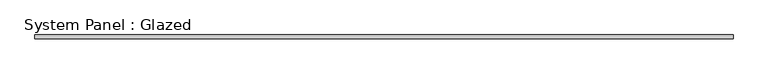
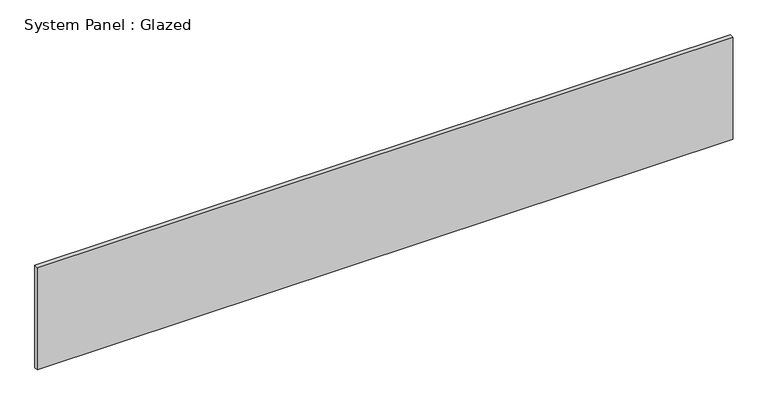
"""IFC4 building model written with IfcOpenShell, lengths in millimetres: plate geometry, System Panel : Glazed."""

from ifc_helpers import new_model, si_unit, origin, origin_with_axes, place, context, project, spatial, polyline, outline, extrude, source, transform, mapped, element, save


def system_panel_glazed_a1088a40(model_context):
    return source(origin(), model_context, "Body", "SweptSolid", [
        extrude(outline(polyline([(2346.325, 24.5), (-2346.325, 24.5), (-2346.325, 49.5), (2346.325, 49.5), (2346.325, 24.5)])), origin_with_axes(), (0.0, 0.0, 1.0), 729.2783674),
    ])


if __name__ == "__main__":
    model = new_model("IFC4")
    model_context = context("Model", 3, world=origin())
    ifc_project = project(units=[si_unit("LENGTHUNIT", "METRE", prefix="MILLI")], contexts=[model_context])
    site = spatial("IfcSite", under=ifc_project)
    building = spatial("IfcBuilding", under=site)
    placement = place(None, origin())
    system_panel_glazed_shape = system_panel_glazed_a1088a40(model_context)
    element("IfcPlate", 1, ObjectType="System Panel : Glazed", at=placement, inside=building, context=model_context, shape_type="MappedRepresentation", body=[
        mapped(system_panel_glazed_shape, transform((0.0, 0.0, 0.0), x_axis=(1.0, 0.0, 0.0), y_axis=(0.0, 1.0, 0.0), z_axis=(0.0, 0.0, 1.0))),
    ])
    save(model, "model.ifc")

# Revit data of these elements
# Type "System Panel : Glazed"
#   Keynote = "H11"
#   Construction Type Id = "GSP4R"
#   Analytic Construction = "1/8 in Pilkington single glazing"
#   Visual Light Transmittance = 0.9
#   Solar Heat Gain Coefficient = 0.86
#   Heat Transfer Coefficient (U) = 6.7069 W/(m²·K)
#   Define Thermal Properties by = 1
# Element 1 (IfcPlate, "System Panel : Glazed")
#   Materials on its faces: "Glass"
# Materials
#   "Glass": class "Glass", colour RGB 0 128 192, transparency 0.9, Description = "Soda Lime Glass", Cost = 0
